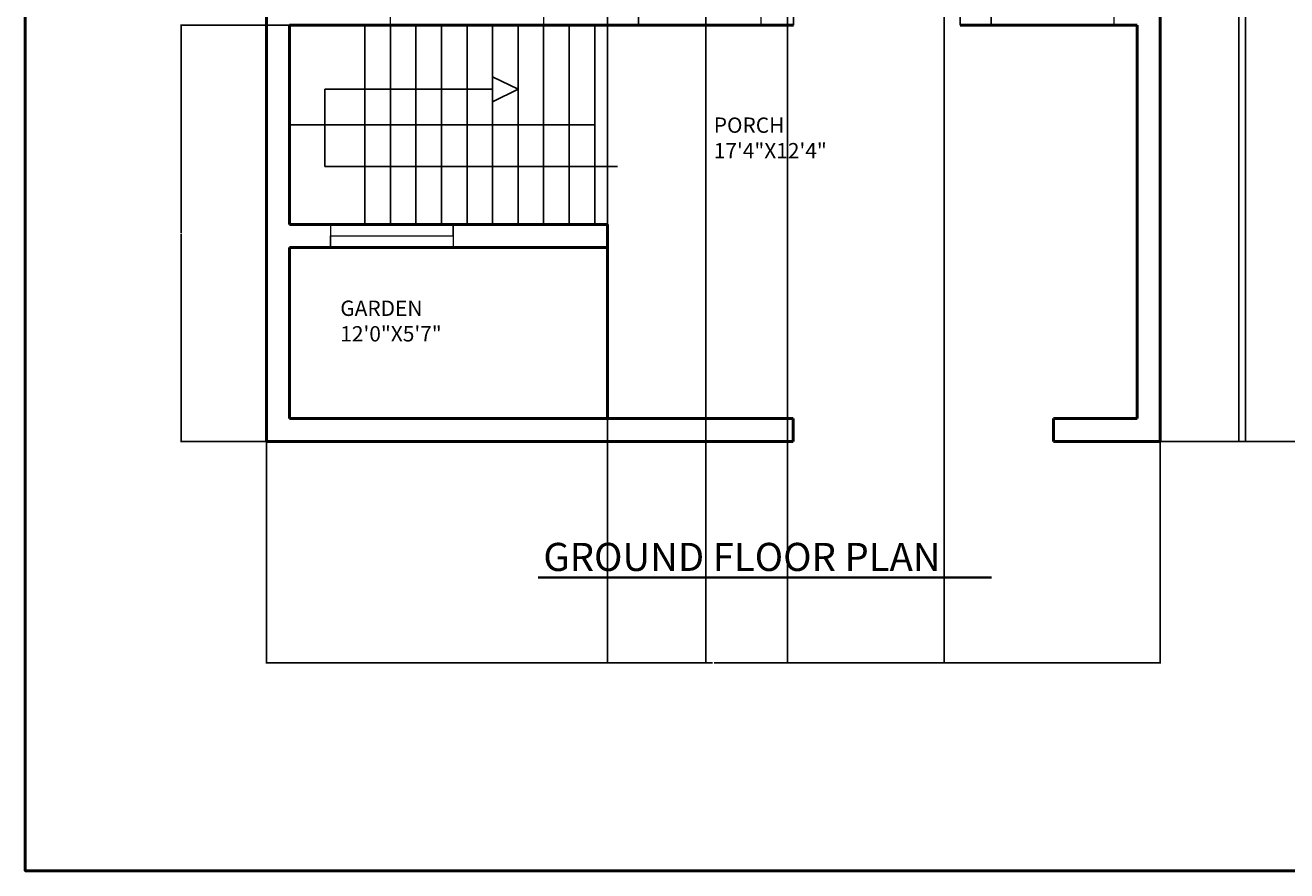
# Model space of a CAD drawing. Units: inches. Extents: x 2268 to 3372, y 1709 to 2892.
# Tile 1 of 6: x 2268 to 2762, y 1709 to 2040. Entities that reach past the tile are written whole.
import ezdxf

# ---------------------------------------------------------------- set-up
doc = ezdxf.new("R2010")
doc.units = ezdxf.units.IN
for name, color, linetype, lineweight in [('A-ANNO-DIMS', 2, 'Continuous', 18), ('A-ANNO-TITL', 7, 'Continuous', 35), ('A-ANNO-TTLB', 7, 'Continuous', 50), ('A-AREA-IDEN', 7, 'Continuous', 18), ('A-DOOR', 3, 'Continuous', 25), ('A-FLOR-STRS', 7, 'Continuous', 25), ('A-GLAZ', 4, 'Continuous', 18), ('A-WALL', 7, 'Continuous', 50)]:
    doc.layers.add(name, color=color, linetype=linetype, lineweight=lineweight)
doc.styles.get("Standard").update_dxf_attribs({"font": 'arial.ttf'})
doc.dimstyles.get("Standard").update_dxf_attribs({"dimtxt": 0.18, "dimasz": 0.18, "dimexe": 0.18, "dimexo": 0.0625, "dimgap": 0.09, "dimtad": 0, "dimtih": 1, "dimtoh": 1, "dimdec": 4, "dimzin": 0, "dimdsep": 46, "dimtxsty": 'Standard', "dimcen": 0.09, "dimadec": 0, "dimazin": 0, "dimtfac": 1, "dimtdec": 4, "dimtofl": 0, "dimtmove": 0, "dimatfit": 3, "dimfxl": 1, "dimtolj": 1, "dimtzin": 0, "dimarcsym": 0})

# ---------------------------------------------------------------- blocks, each defined once
blk = doc.blocks.new('DOOR-ENTRY-PAIR')
for p, q in [((2, 4.5), (2, 52.5)), ((63.28, 40.5), (63.28, 52.5)), ((63.28, 4.5), (63.28, 40.5)), ((0, 9), (0, 0)), ((65.28, 9), (65.28, 0)), ((0, 0), (0, 4.5)), ((0, 4.5), (2, 4.5)), ((65.28, 4.5), (63.28, 4.5)), ((65.28, 0), (65.28, 4.5))]:
    blk.add_line(p, q)
for centre, radius, start, end in [((2, 21.15), 31.35, 16.9315, 90), ((63.59, 18.92), 33.58, 90.5202, 160.2273)]:
    blk.add_arc(centre, radius, start, end)
blk = doc.blocks.new('WIN-48')
for p, q in [((0, 9), (0, 0)), ((48, 4.5), (48, 9)), ((48, 9), (48, 0)), ((0, 0), (0, 4.5)), ((0, 4.5), (48, 4.5))]:
    blk.add_line(p, q)
blk = doc.blocks.new('WIN-60')
for p, q in [((0, 60), (9, 60)), ((9, 60), (4.5, 60)), ((4.5, 60), (4.5, 0)), ((9, 0), (0, 0)), ((4.5, 0), (9, 0))]:
    blk.add_line(p, q)
blk = doc.blocks.new('STAIR-FRONT-RETURN')
for p, q in [((29.53, 0), (29.53, 78)), ((39.53, 0), (39.53, 78)), ((49.53, 0), (49.53, 78)), ((59.53, 0), (59.53, 78)), ((69.53, 0), (69.53, 78)), ((79.53, 0), (79.53, 78)), ((89.53, 0), (89.53, 78)), ((99.53, 0), (99.53, 78)), ((109.53, 0), (109.53, 78)), ((119.53, 0), (119.53, 78)), ((89.53, 52.91), (79.53, 57.75)), ((79.53, 57.75), (79.53, 48.01)), ((13.79, 22.73), (13.79, 52.91)), ((13.79, 52.91), (79.53, 52.91)), ((79.53, 48.01), (89.53, 52.91)), ((0, 39), (119.53, 39)), ((119.53, 39), (119.53, 0)), ((128.5, 22.73), (13.79, 22.73))]:
    blk.add_line(p, q)
blk = doc.blocks.new('*D76')
at = {"layer": 'A-ANNO-DIMS', "color": 0, "lineweight": -2, "transparency": 16777216}
for p, q in [((2362.89, 1877.11), (2362.89, 1790.27)), ((2712.89, 1877.11), (2712.89, 1790.27)), ((2363.07, 1790.45), (2537.61, 1790.45)), ((2712.71, 1790.45), (2538.18, 1790.45))]:
    blk.add_line(p, q, dxfattribs=at)
at = {"layer": 'A-ANNO-DIMS', "color": 0, "transparency": 16777216}
for points in [[(2363.07, 1790.48), (2363.07, 1790.42), (2362.89, 1790.45)], [(2712.71, 1790.48), (2712.71, 1790.42), (2712.89, 1790.45)]]:
    blk.add_solid(points, dxfattribs=at)
at = {"layer": 'Defpoints', "color": 0, "transparency": 16777216}
for p in [(2362.89, 1877.18), (2712.89, 1877.18), (2712.89, 1790.45)]:
    blk.add_point(p, dxfattribs=at)
at = {"layer": 'A-ANNO-DIMS', "color": 0, "transparency": 16777216, "insert": (2537.89, 1790.45), "char_height": 0.18, "attachment_point": 5}
blk.add_mtext('\\A1;350', dxfattribs=at)
blk = doc.blocks.new('*D77')
at = {"layer": 'A-ANNO-DIMS', "color": 0, "lineweight": -2, "transparency": 16777216}
for p, q in [((2712.96, 2463.18), (2746.52, 2463.18)), ((2746.34, 2463), (2746.34, 2170.36)), ((2746.34, 1877.36), (2746.34, 2169.99)), ((2712.96, 1877.18), (2746.52, 1877.18))]:
    blk.add_line(p, q, dxfattribs=at)
at = {"layer": 'A-ANNO-DIMS', "color": 0, "transparency": 16777216}
for points in [[(2746.31, 2463), (2746.37, 2463), (2746.34, 2463.18)], [(2746.31, 1877.36), (2746.37, 1877.36), (2746.34, 1877.18)]]:
    blk.add_solid(points, dxfattribs=at)
at = {"layer": 'Defpoints', "color": 0, "transparency": 16777216}
for p in [(2712.89, 2463.18), (2746.34, 2463.18), (2712.89, 1877.18)]:
    blk.add_point(p, dxfattribs=at)
at = {"layer": 'A-ANNO-DIMS', "color": 0, "transparency": 16777216, "insert": (2746.34, 2170.18), "char_height": 0.18, "attachment_point": 5}
blk.add_mtext('\\A1;586', dxfattribs=at)
blk = doc.blocks.new('*D81')
at = {"layer": 'A-ANNO-DIMS', "color": 0, "lineweight": -2, "transparency": 16777216}
for p, q in [((2496.39, 2382.11), (2496.39, 1790.27)), ((2534.88, 2377.61), (2534.88, 1790.27)), ((2496.57, 1790.45), (2515.17, 1790.45)), ((2534.7, 1790.45), (2516.1, 1790.45))]:
    blk.add_line(p, q, dxfattribs=at)
at = {"layer": 'A-ANNO-DIMS', "color": 0, "transparency": 16777216}
for points in [[(2496.57, 1790.48), (2496.57, 1790.42), (2496.39, 1790.45)], [(2534.7, 1790.48), (2534.7, 1790.42), (2534.88, 1790.45)]]:
    blk.add_solid(points, dxfattribs=at)
at = {"layer": 'Defpoints', "color": 0, "transparency": 16777216}
for p in [(2496.39, 2382.18), (2534.88, 2377.68), (2534.88, 1790.45)]:
    blk.add_point(p, dxfattribs=at)
at = {"layer": 'A-ANNO-DIMS', "color": 0, "transparency": 16777216, "insert": (2515.64, 1790.45), "char_height": 0.18, "attachment_point": 5}
blk.add_mtext('\\A1;38.486', dxfattribs=at)
blk = doc.blocks.new('*D82')
at = {"layer": 'A-ANNO-DIMS', "color": 0, "lineweight": -2, "transparency": 16777216}
for p, q in [((2566.89, 2389.61), (2566.89, 1790.27)), ((2628.3, 2389.61), (2628.3, 1790.27)), ((2567.07, 1790.45), (2597.22, 1790.45)), ((2628.12, 1790.45), (2597.98, 1790.45))]:
    blk.add_line(p, q, dxfattribs=at)
at = {"layer": 'A-ANNO-DIMS', "color": 0, "transparency": 16777216}
for points in [[(2567.07, 1790.48), (2567.07, 1790.42), (2566.89, 1790.45)], [(2628.12, 1790.48), (2628.12, 1790.42), (2628.3, 1790.45)]]:
    blk.add_solid(points, dxfattribs=at)
at = {"layer": 'Defpoints', "color": 0, "transparency": 16777216}
for p in [(2566.89, 2389.68), (2628.3, 2389.68), (2628.3, 1790.45)]:
    blk.add_point(p, dxfattribs=at)
at = {"layer": 'A-ANNO-DIMS', "color": 0, "transparency": 16777216, "insert": (2597.6, 1790.45), "char_height": 0.18, "attachment_point": 5}
blk.add_mtext('\\A1;61.41', dxfattribs=at)
blk = doc.blocks.new('*D83')
at = {"layer": 'A-ANNO-DIMS', "color": 0, "lineweight": -2, "transparency": 16777216}
for p, q in [((2371.83, 2040.18), (2329.26, 2040.18)), ((2329.44, 2040), (2329.44, 1958.86)), ((2329.44, 1877.36), (2329.44, 1958.49)), ((2362.83, 1877.18), (2329.26, 1877.18))]:
    blk.add_line(p, q, dxfattribs=at)
at = {"layer": 'A-ANNO-DIMS', "color": 0, "transparency": 16777216}
for points in [[(2329.41, 2040), (2329.47, 2040), (2329.44, 2040.18)], [(2329.41, 1877.36), (2329.47, 1877.36), (2329.44, 1877.18)]]:
    blk.add_solid(points, dxfattribs=at)
at = {"layer": 'Defpoints', "color": 0, "transparency": 16777216}
for p in [(2329.44, 2040.18), (2371.89, 2040.18), (2362.89, 1877.18)]:
    blk.add_point(p, dxfattribs=at)
at = {"layer": 'A-ANNO-DIMS', "color": 0, "transparency": 16777216, "insert": (2329.44, 1958.68), "char_height": 0.18, "attachment_point": 5}
blk.add_mtext('\\A1;163', dxfattribs=at)
blk = doc.blocks.new('*D93')
at = {"layer": 'A-ANNO-DIMS', "color": 0, "lineweight": -2, "transparency": 16777216}
for p, q in [((2812.94, 2463.18), (2743.52, 2463.18)), ((2743.7, 2463), (2743.7, 2170.36)), ((2743.7, 1877.36), (2743.7, 2169.99)), ((2812.94, 1877.18), (2743.52, 1877.18))]:
    blk.add_line(p, q, dxfattribs=at)
at = {"layer": 'A-ANNO-DIMS', "color": 0, "transparency": 16777216}
for points in [[(2743.67, 2463), (2743.73, 2463), (2743.7, 2463.18)], [(2743.67, 1877.36), (2743.73, 1877.36), (2743.7, 1877.18)]]:
    blk.add_solid(points, dxfattribs=at)
at = {"layer": 'Defpoints', "color": 0, "transparency": 16777216}
for p in [(2743.7, 2463.18), (2813, 2463.18), (2813, 1877.18)]:
    blk.add_point(p, dxfattribs=at)
at = {"layer": 'A-ANNO-DIMS', "color": 0, "transparency": 16777216, "insert": (2743.7, 2170.18), "char_height": 0.18, "attachment_point": 5}
blk.add_mtext('\\A1;586', dxfattribs=at)

msp = doc.modelspace()

# ---------------------------------------------------------------- linework, layer by layer
at = {"layer": 'A-ANNO-TITL'}
msp.add_line((2469.2419, 1823.9038), (2646.778, 1823.9038), dxfattribs=at)
msp.add_line((2469.2419, 1823.9038), (2646.778, 1823.9038), dxfattribs=at)
at = {"layer": 'A-ANNO-TTLB'}
msp.add_lwpolyline([(2268.3884, 2892.2471), (3372.3464, 2892.2471), (3372.3464, 1709.0755), (2268.3884, 1709.0755)], close=True, dxfattribs=at)
at = {"layer": 'A-WALL'}
for p, q in [((2362.8943, 2463.1756), (2362.8943, 1877.1756)), ((2362.8943, 2463.1756), (2362.8943, 1877.1756)), ((2712.8943, 2463.1756), (2712.8943, 1877.1756)), ((2712.8943, 2463.1756), (2712.8943, 1877.1756)), ((2371.8943, 2040.1756), (2491.8943, 2040.1756)), ((2371.8943, 2040.1756), (2371.8943, 1962.1756)), ((2371.8943, 2040.1756), (2491.8943, 2040.1756)), ((2371.8943, 2040.1756), (2371.8943, 1962.1756)), ((2491.8943, 2040.1756), (2496.3943, 2040.1756)), ((2491.8943, 2040.1756), (2496.3943, 2040.1756)), ((2496.3943, 2040.1756), (2569.2467, 2040.1756)), ((2496.3943, 2040.1756), (2569.2467, 2040.1756)), ((2634.5318, 2040.1756), (2703.8943, 2040.1756)), ((2634.5318, 2040.1756), (2703.8943, 2040.1756)), ((2703.8943, 2040.1756), (2703.8943, 1886.1756)), ((2703.8943, 2040.1756), (2703.8943, 1886.1756)), ((2371.8943, 1962.1756), (2491.8943, 1962.1756)), ((2371.8943, 1962.1756), (2491.8943, 1962.1756)), ((2491.8943, 1962.1756), (2491.8943, 1962.1756)), ((2491.8943, 1962.1756), (2496.3943, 1962.1756)), ((2491.8943, 1962.1756), (2491.8943, 1962.1756)), ((2491.8943, 1962.1756), (2496.3943, 1962.1756)), ((2496.3943, 1962.1756), (2496.3943, 1886.1756)), ((2496.3943, 1962.1756), (2496.3943, 1886.1756)), ((2371.8943, 1953.1756), (2491.8943, 1953.1756)), ((2371.8943, 1953.1756), (2371.8943, 1886.1756)), ((2371.8943, 1953.1756), (2491.8943, 1953.1756)), ((2371.8943, 1953.1756), (2371.8943, 1886.1756)), ((2491.8943, 1953.1756), (2496.3943, 1953.1756)), ((2491.8943, 1953.1756), (2496.3943, 1953.1756)), ((2371.8943, 1886.1756), (2491.8943, 1886.1756)), ((2371.8943, 1886.1756), (2491.8943, 1886.1756)), ((2491.8943, 1886.1756), (2496.3943, 1886.1756)), ((2491.8943, 1886.1756), (2496.3943, 1886.1756)), ((2569.1319, 1886.1756), (2496.3943, 1886.1756)), ((2569.1319, 1886.1756), (2496.3943, 1886.1756)), ((2569.1319, 1877.1756), (2569.1319, 1886.1756)), ((2569.1319, 1877.1756), (2569.1319, 1886.1756)), ((2671.0939, 1886.1756), (2703.8943, 1886.1756)), ((2703.8943, 1886.1756), (2671.0939, 1886.1756)), ((2671.0939, 1886.1756), (2671.0939, 1877.1756)), ((2671.0939, 1886.1756), (2703.8943, 1886.1756)), ((2703.8943, 1886.1756), (2671.0939, 1886.1756)), ((2671.0939, 1886.1756), (2671.0939, 1877.1756)), ((2371.8943, 1877.1756), (2362.8943, 1877.1756)), ((2371.8943, 1877.1756), (2362.8943, 1877.1756)), ((2371.8943, 1877.1756), (2491.8943, 1877.1756)), ((2371.8943, 1877.1756), (2491.8943, 1877.1756)), ((2496.3943, 1877.1756), (2491.8943, 1877.1756)), ((2496.3943, 1877.1756), (2491.8943, 1877.1756)), ((2496.3943, 1877.1756), (2569.1319, 1877.1756)), ((2496.3943, 1877.1756), (2569.1319, 1877.1756)), ((2671.0939, 1877.1756), (2703.8943, 1877.1756)), ((2671.0939, 1877.1756), (2703.8943, 1877.1756)), ((2703.8943, 1877.1756), (2712.8943, 1877.1756)), ((2703.8943, 1877.1756), (2712.8943, 1877.1756))]:
    msp.add_line(p, q, dxfattribs=at)

# ---------------------------------------------------------------- block references
at = {"layer": 'A-DOOR'}
msp.add_blockref('DOOR-ENTRY-PAIR', (2569.247, 2040.176), dxfattribs=at)
msp.add_blockref('DOOR-ENTRY-PAIR', (2569.247, 2040.176), dxfattribs=at)
at = {"layer": 'A-FLOR-STRS'}
msp.add_blockref('STAIR-FRONT-RETURN', (2371.894, 1962.176), dxfattribs=at)
msp.add_blockref('STAIR-FRONT-RETURN', (2371.894, 1962.176), dxfattribs=at)
at = {"layer": 'A-GLAZ'}
for rotation in [89.99999999999905, 89.9999999999979]:
    msp.add_blockref('WIN-60', (2471.4241, 2040.1753), dxfattribs=dict(at, rotation=rotation))
for p in [(2508.522, 2040.176), (2508.522, 2040.176), (2646.685, 2040.176), (2646.685, 2040.176), (2387.9738, 1953.176), (2387.9738, 1953.176)]:
    msp.add_blockref('WIN-48', p, dxfattribs=at)

# ---------------------------------------------------------------- texts
at = {"layer": 'A-ANNO-TITL', "insert": (2471.2955, 1837.4758), "char_height": 11, "attachment_point": 1}
msp.add_mtext_dynamic_manual_height_columns('GROUND FLOOR PLAN', width=367.537045, gutter_width=12.5, heights=[0], dxfattribs=at)
at = {"layer": 'A-AREA-IDEN', "char_height": 6, "attachment_point": 1}
for s, width, insert in [('PORCH\\P17\'4"X12\'4"', 89.961396, (2538.049, 2004.0476)), ('PORCH\\P17\'4"X12\'4"', 89.961396, (2538.049, 2004.0476)), ('GARDEN\\P12\'0"X5\'7"', 89.737714, (2391.7812, 1932.3469)), ('GARDEN\\P12\'0"X5\'7"', 89.737714, (2391.7812, 1932.3469))]:
    msp.add_mtext_dynamic_manual_height_columns(s, width=width, gutter_width=12.5, heights=[0], dxfattribs=dict(at, insert=insert))

# ---------------------------------------------------------------- dimensions: what is measured, and where the dimension line sits
at = {"layer": 'A-ANNO-DIMS'}
for base, p1, p2, picture, middle in [((2746.3443, 2463.1756), (2712.8943, 1877.1756), (2712.8943, 2463.1756), '*D77', (2746.3443, 2170.1756)), ((2743.7041, 2463.1756), (2813.001, 1877.1756), (2813.001, 2463.1756), '*D93', (2743.7041, 2170.1756)), ((2329.4443, 2040.1756), (2362.8943, 1877.1756), (2371.8943, 2040.1756), '*D83', (2329.4443, 1958.6756))]:
    dim = msp.add_linear_dim(base=base, p1=p1, p2=p2, angle=90, dimstyle='Standard', override={"dimdec": 0, "dimlfac": 1, "dimrnd": 0, "dimzin": 0, "dimdsep": 46, "dimlunit": 2}, dxfattribs=at)
    dim.commit()
    dim.dimension.update_dxf_attribs({"geometry": picture, "text_midpoint": middle})
for base, p1, p2, override, picture, middle in [((2628.3027, 1790.4538), (2566.8943, 2389.6756), (2628.3027, 2389.6756), {"dimdec": 2, "dimlfac": 1, "dimrnd": 0, "dimzin": 0, "dimdsep": 46, "dimlunit": 2}, '*D82', (2597.5985, 1790.4538)), ((2534.8799, 1790.4538), (2496.3943, 2382.1756), (2534.8799, 2377.6756), {"dimdec": 3, "dimlfac": 1, "dimrnd": 0, "dimzin": 0, "dimdsep": 46, "dimlunit": 2}, '*D81', (2515.6371, 1790.4538)), ((2712.8943, 1790.4538), (2362.8943, 1877.1756), (2712.8943, 1877.1756), {"dimdec": 0, "dimlfac": 1, "dimrnd": 0, "dimzin": 0, "dimdsep": 46, "dimlunit": 2}, '*D76', (2537.8943, 1790.4538))]:
    dim = msp.add_linear_dim(base=base, p1=p1, p2=p2, dimstyle='Standard', override=override, dxfattribs=at)
    dim.commit()
    dim.dimension.update_dxf_attribs({"geometry": picture, "text_midpoint": middle})

doc.saveas('drawing.dxf')
